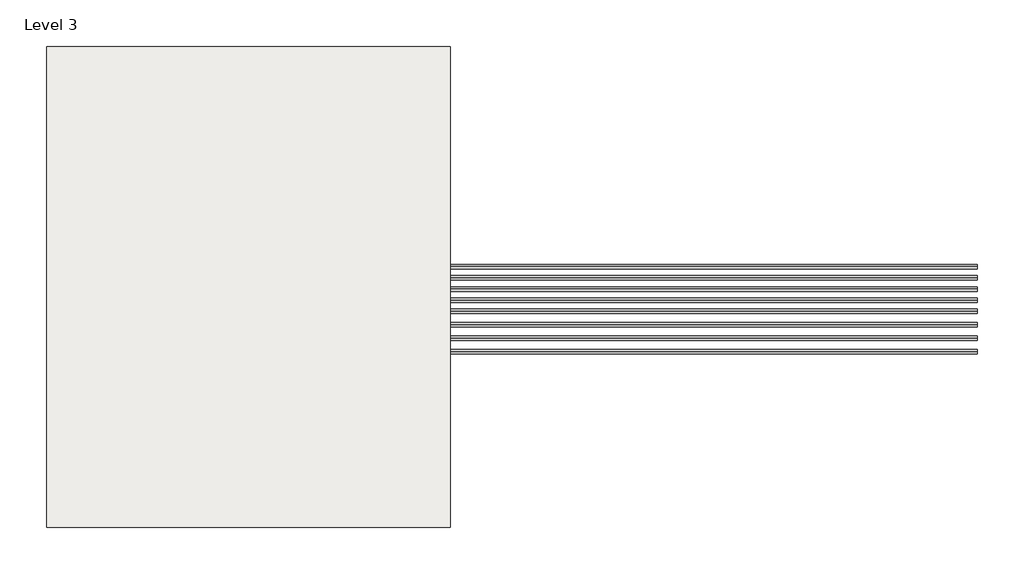
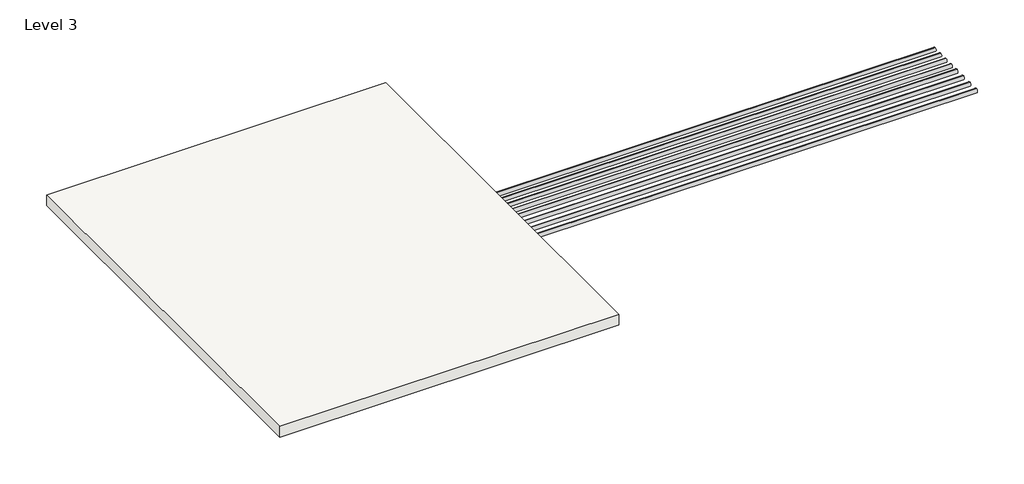
# One storey: 1 covering, 1 proxy.
"""IFC4 building model written with IfcOpenShell, lengths in millimetres."""

from ifc_helpers import new_model, si_unit, frame, origin, place, context, project, spatial, polyline, outline, extrude, transform, mapped, element, save
from components import generic_models_11_generic_models_11_8b992ad3

model = new_model("IFC4")

# Units and contexts
model_context = context("Model", 3, world=origin())
ifc_project = project(units=[si_unit("LENGTHUNIT", "METRE", prefix="MILLI")], contexts=[model_context])

# Site, building, storey
site = spatial("IfcSite", under=ifc_project)
building = spatial("IfcBuilding", under=site)
storey = spatial("IfcBuildingStorey", under=building, Name="Level 3", Elevation=10058.4)

# Proxy
placement = place(None, origin())
generic_models_11_generic_models_11_shape = generic_models_11_generic_models_11_8b992ad3(model_context)
element("IfcBuildingElementProxy", 1, Name="Generic Models 11 : Generic Models 11", ObjectType="Generic Models 11 : Generic Models 11", at=placement, inside=storey, context=model_context, shape_type="MappedRepresentation", body=[
    mapped(generic_models_11_generic_models_11_shape, transform((0.0, 0.0, 0.0), x_axis=(1.0, 0.0, 0.0), y_axis=(0.0, 1.0, 0.0), z_axis=(0.0, 0.0, 1.0))),
])

# Covering
element("IfcCovering", 2, ObjectType="300mm_Generic 2 6\"", at=placement, inside=storey, context=model_context, shape_type="SweptSolid", body=[
    extrude(outline(polyline([(-10825.2463366, 968.9684231), (-10825.2463366, -4479.5968048), (-15397.2463366, -4479.5968048), (-15397.2463366, 968.9684231), (-10825.2463366, 968.9684231)])), frame((0.0, 0.0, 10058.4), z_axis=(0.0, 0.0, 1.0), x_axis=(1.0, 0.0, 0.0)), (0.0, 0.0, 1.0), 152.4),
])

save(model, "model.ifc")

# Revit data of these elements
# Type "300mm_Generic 2 6\""
#   built-in parameter 1002203 = 1 (stored number, unit not read)
#   built-in parameter 1002202 = 1 (stored number, unit not read)
#   Layers, outside or top first: 0' - 6" no material (function 1)
# Element 1 (IfcBuildingElementProxy, "Generic Models 11 : Generic Models 11")
#   Phase Created = New Construction
# Element 2 (IfcCovering, "300mm_Generic 2 6\"")
#   Height Offset From Level = 0' - 0"
#   Phase Created = New Construction
#   Materials on its faces: "Default"
# Materials
#   "Default": colour RGB 127 127 127, transparency 0, Cost = 0
